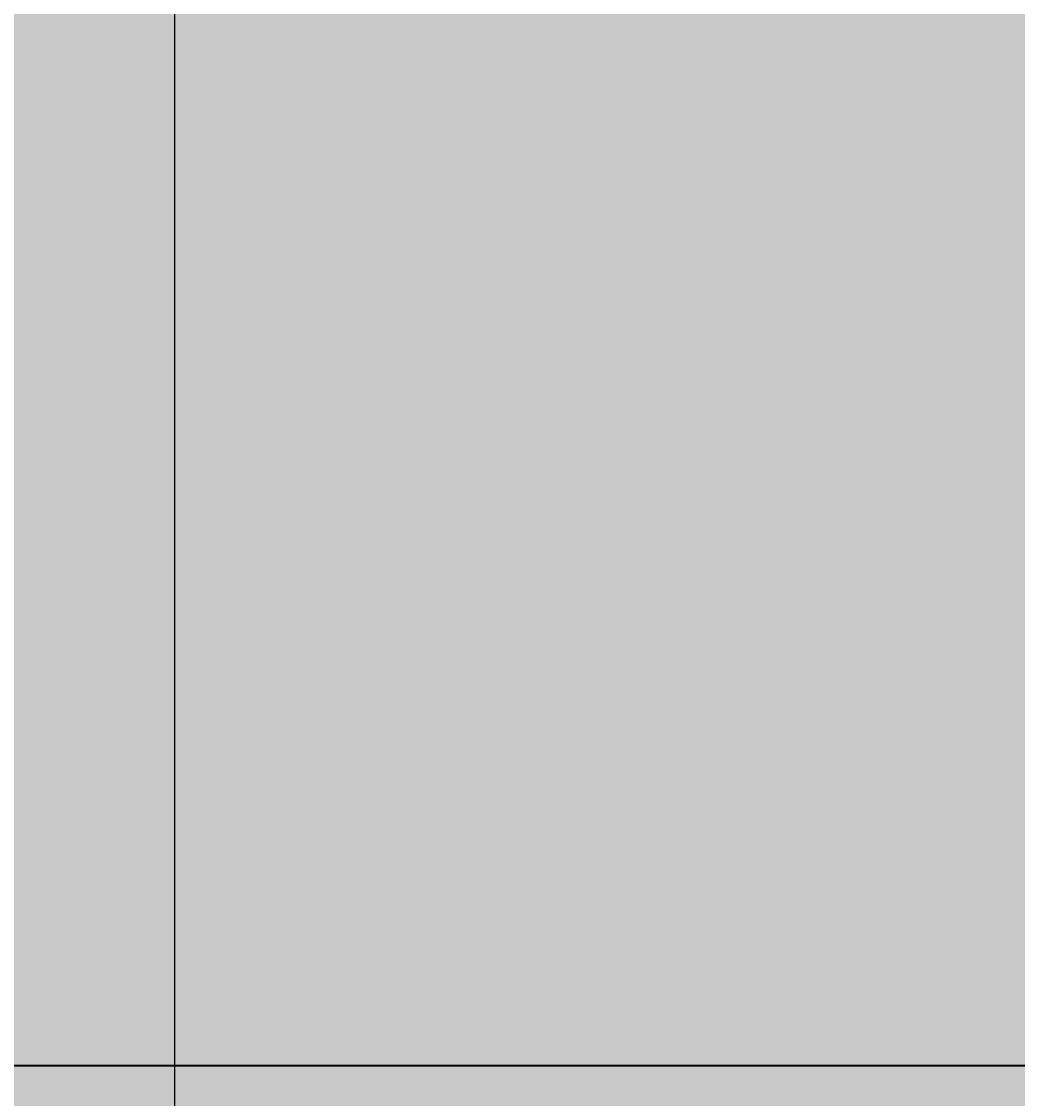
# Model space of a CAD drawing. Units: feet. Extents: x 2695 to 2912, y 795 to 1139.
# Tile 70 of 83: x 2805 to 2840, y 1062 to 1100. Entities that reach past the tile are written whole.
import ezdxf

# ---------------------------------------------------------------- set-up
doc = ezdxf.new("R2010")
doc.units = ezdxf.units.FT
for name, color, linetype, lineweight in [('A-ANNO-DIMS', 2, 'Continuous', 18), ('A-ELEV', 7, 'Continuous', 35), ('A-ELEV-PATT', 252, 'Continuous', 13)]:
    doc.layers.add(name, color=color, linetype=linetype, lineweight=lineweight)
doc.styles.get("Standard").update_dxf_attribs({"font": 'arial.ttf'})
doc.dimstyles.get("Standard").update_dxf_attribs({"dimtxt": 0.18, "dimasz": 0.18, "dimexe": 0.18, "dimexo": 0.0625, "dimgap": 0.09, "dimtad": 0, "dimtih": 1, "dimtoh": 1, "dimdec": 1, "dimzin": 0, "dimdsep": 46, "dimlunit": 3, "dimtxsty": 'Standard', "dimcen": 0.09, "dimadec": 0, "dimazin": 0, "dimtfac": 1, "dimtdec": 1, "dimtofl": 0, "dimtmove": 0, "dimatfit": 3, "dimfxl": 1, "dimtolj": 1, "dimtzin": 0, "dimarcsym": 0})

# ---------------------------------------------------------------- blocks, each defined once
blk = doc.blocks.new('*D10')
at = {"layer": 'A-ANNO-DIMS', "color": 0, "lineweight": -2, "transparency": 16777216}
for p, q in [((2778.034, 1020.886), (2778.034, 1138.886)), ((2778.214, 1138.706), (2810.411, 1138.706)), ((2843.395, 1138.706), (2811.198, 1138.706)), ((2843.575, 1020.886), (2843.575, 1138.886))]:
    blk.add_line(p, q, dxfattribs=at)
at = {"layer": 'A-ANNO-DIMS', "color": 0, "transparency": 16777216}
for points in [[(2778.214, 1138.736), (2778.214, 1138.676), (2778.034, 1138.706)], [(2843.395, 1138.736), (2843.395, 1138.676), (2843.575, 1138.706)]]:
    blk.add_solid(points, dxfattribs=at)
at = {"layer": 'Defpoints', "color": 0, "transparency": 16777216}
for p in [(2843.575, 1138.706), (2778.034, 1020.824), (2843.575, 1020.824)]:
    blk.add_point(p, dxfattribs=at)
at = {"layer": 'A-ANNO-DIMS', "color": 0, "transparency": 16777216, "insert": (2810.805, 1138.706), "char_height": 0.18, "attachment_point": 5}
blk.add_mtext('\\A1;65.54', dxfattribs=at)
blk = doc.blocks.new('*D49')
at = {"layer": 'A-ANNO-DIMS', "color": 0, "lineweight": -2, "transparency": 16777216}
for p, q in [((2772.522, 972.03), (2772.522, 1138.886)), ((2772.702, 1138.706), (2790.888, 1138.706)), ((2809.861, 1138.706), (2791.674, 1138.706)), ((2810.041, 972.03), (2810.041, 1138.886))]:
    blk.add_line(p, q, dxfattribs=at)
at = {"layer": 'A-ANNO-DIMS', "color": 0, "transparency": 16777216}
for points in [[(2772.702, 1138.736), (2772.702, 1138.676), (2772.522, 1138.706)], [(2809.861, 1138.736), (2809.861, 1138.676), (2810.041, 1138.706)]]:
    blk.add_solid(points, dxfattribs=at)
at = {"layer": 'Defpoints', "color": 0, "transparency": 16777216}
for p in [(2810.041, 1138.706), (2772.522, 971.967), (2810.041, 971.967)]:
    blk.add_point(p, dxfattribs=at)
at = {"layer": 'A-ANNO-DIMS', "color": 0, "transparency": 16777216, "insert": (2791.281, 1138.706), "char_height": 0.18, "attachment_point": 5}
blk.add_mtext('\\A1;37.52', dxfattribs=at)
blk = doc.blocks.new('*D50')
at = {"layer": 'A-ANNO-DIMS', "color": 0, "lineweight": -2, "transparency": 16777216}
for p, q in [((2810.041, 972.03), (2810.041, 1138.886)), ((2810.221, 1138.706), (2848.721, 1138.706)), ((2888.008, 1138.706), (2849.508, 1138.706)), ((2888.188, 972.03), (2888.188, 1138.886))]:
    blk.add_line(p, q, dxfattribs=at)
at = {"layer": 'A-ANNO-DIMS', "color": 0, "transparency": 16777216}
for points in [[(2810.221, 1138.736), (2810.221, 1138.676), (2810.041, 1138.706)], [(2888.008, 1138.736), (2888.008, 1138.676), (2888.188, 1138.706)]]:
    blk.add_solid(points, dxfattribs=at)
at = {"layer": 'Defpoints', "color": 0, "transparency": 16777216}
for p in [(2888.188, 1138.706), (2810.041, 971.967), (2888.188, 971.967)]:
    blk.add_point(p, dxfattribs=at)
at = {"layer": 'A-ANNO-DIMS', "color": 0, "transparency": 16777216, "insert": (2849.114, 1138.706), "char_height": 0.18, "attachment_point": 5}
blk.add_mtext('\\A1;78.15', dxfattribs=at)

msp = doc.modelspace()

# ---------------------------------------------------------------- hatches: boundary and pattern name
at = {"layer": 'A-ELEV-PATT'}
h = msp.add_hatch(color=256, dxfattribs=at)
h.set_gradient(color1=(255, 255, 255), tint=1)
h.paths.add_polyline_path([(2770.6361, 1122.9306), (2710.6361, 1122.9306), (2710.6361, 1118.4096), (2770.6361, 1118.4096)])
h.paths.add_polyline_path([(2890.6361, 1107.8588), (2770.6361, 1107.8588), (2770.6361, 1103.3378), (2890.6361, 1103.3378)])
h.paths.add_polyline_path([(2890.6361, 1062.9306), (2710.6361, 1062.9306), (2710.6361, 1056.9306), (2710.6361, 936.9306), (2710.6361, 924.3105), (2716.5358, 924.3105), (2890.6361, 924.3105), (2890.6361, 936.9306), (2715.8852, 936.9306), (2715.8852, 1050.3105), (2890.6361, 1050.3105)])
h.paths.add_polyline_path([(2716.5358, 924.3105), (2710.6361, 924.3105), (2710.6361, 810.9306), (2716.5358, 810.9306)])
h = msp.add_hatch(color=256, dxfattribs=at)
h.set_gradient(color1=(147, 149, 152), color2=(147, 149, 152), tint=1)
h.paths.add_polyline_path([(2770.6361, 1118.4096), (2710.6361, 1118.4096), (2710.6361, 1062.9306), (2770.6361, 1062.9306)])
h.paths.add_polyline_path([(2890.6361, 1103.3378), (2770.6361, 1103.3378), (2770.6361, 1062.9306), (2890.6361, 1062.9306)])
h.paths.add_polyline_path([(2730.7081, 1048.1052), (2755.1125, 1048.1052), (2755.1125, 936.9306), (2770.6361, 936.9306), (2770.6361, 1050.3105), (2715.8852, 1050.3105), (2715.8852, 936.9306), (2730.7081, 936.9306)])
h.paths.add_polyline_path([(2890.6361, 1050.3105), (2770.6361, 1050.3105), (2770.6361, 971.9673), (2778.0341, 971.9673), (2778.0341, 1020.8235), (2843.575, 1020.8235), (2843.575, 971.9673), (2890.6361, 971.9673)])
h.paths.add_polyline_path([(2888.1882, 970.7156), (2843.575, 970.7156), (2843.575, 964.8267), (2888.1882, 964.8267)])
h.paths.add_polyline_path([(2888.1882, 964.1328), (2843.575, 964.1328), (2843.575, 956.614), (2888.1882, 956.614)])
h.paths.add_polyline_path([(2888.1882, 955.9202), (2843.575, 955.9202), (2843.575, 949.2892), (2888.1882, 949.2892)])
h.paths.add_polyline_path([(2888.1882, 948.5954), (2843.575, 948.5954), (2843.575, 941.3507), (2888.1882, 941.3507)])
h.paths.add_polyline_path([(2888.1882, 940.6569), (2843.575, 940.6569), (2843.575, 936.9306), (2888.1882, 936.9306)])
h.paths.add_polyline_path([(2890.6361, 970.7156), (2888.9368, 970.7156), (2888.9368, 964.8267), (2890.6361, 964.8267)])
h.paths.add_polyline_path([(2890.6361, 964.1328), (2888.9368, 964.1328), (2888.9368, 956.614), (2890.6361, 956.614)])
h.paths.add_polyline_path([(2890.6361, 955.9202), (2888.9368, 955.9202), (2888.9368, 949.2892), (2890.6361, 949.2892)])
h.paths.add_polyline_path([(2890.6361, 940.6569), (2888.9368, 940.6569), (2888.9368, 936.9306), (2890.6361, 936.9306)])
h.paths.add_polyline_path([(2890.6361, 948.5954), (2888.9368, 948.5954), (2888.9368, 941.3507), (2890.6361, 941.3507)])
h.paths.add_polyline_path([(2772.5216, 970.7156), (2770.6361, 970.7156), (2770.6361, 964.8267), (2772.5216, 964.8267)])
h.paths.add_polyline_path([(2772.5216, 964.1328), (2770.6361, 964.1328), (2770.6361, 956.614), (2772.5216, 956.614)])
h.paths.add_polyline_path([(2772.5216, 955.9202), (2770.6361, 955.9202), (2770.6361, 949.2892), (2772.5216, 949.2892)])
h.paths.add_polyline_path([(2772.5216, 948.5954), (2770.6361, 948.5954), (2770.6361, 941.3507), (2772.5216, 941.3507)])
h.paths.add_polyline_path([(2772.5216, 940.6569), (2770.6361, 940.6569), (2770.6361, 936.9306), (2772.5216, 936.9306)])
h.paths.add_polyline_path([(2778.0341, 940.6569), (2773.2702, 940.6569), (2773.2702, 936.9306), (2778.0341, 936.9306)])
h.paths.add_polyline_path([(2778.0341, 970.7156), (2773.2702, 970.7156), (2773.2702, 964.8267), (2778.0341, 964.8267)])
h.paths.add_polyline_path([(2778.0341, 964.1328), (2773.2702, 964.1328), (2773.2702, 956.614), (2778.0341, 956.614)])
h.paths.add_polyline_path([(2778.0341, 955.9202), (2773.2702, 955.9202), (2773.2702, 949.2892), (2778.0341, 949.2892)])
h.paths.add_polyline_path([(2778.0341, 948.5954), (2773.2702, 948.5954), (2773.2702, 941.3507), (2778.0341, 941.3507)])
h.paths.add_polyline_path([(2810.0407, 940.6569), (2780.0341, 940.6569), (2780.0341, 936.9306), (2810.0407, 936.9306)])
h.paths.add_polyline_path([(2890.6361, 924.3105), (2770.6361, 924.3105), (2770.6361, 810.9306), (2773.5029, 810.9306), (2773.5029, 905.5143), (2805.9398, 905.5143), (2838.3767, 905.5143), (2838.3767, 810.9306), (2890.6361, 810.9306)])
h = msp.add_hatch(color=256, dxfattribs=at)
h.set_gradient(color1=(199, 200, 202), color2=(213, 227, 240), centered=1)
h.paths.add_polyline_path([(2890.6361, 1103.3378), (2770.6361, 1103.3378), (2770.6361, 1062.9306), (2890.6361, 1062.9306)])

# ---------------------------------------------------------------- linework, layer by layer
at = {"layer": 'A-ELEV'}
for q in [(2890.6361, 1062.9306), (2895.4694, 1062.9306)]:
    msp.add_line((2710.6361, 1062.9306), q, dxfattribs=at)

# ---------------------------------------------------------------- dimensions: what is measured, and where the dimension line sits
at = {"layer": 'A-ANNO-DIMS'}
for base, p1, p2, picture, middle in [((2810.0407, 1138.7056), (2772.5216, 971.9673), (2810.0407, 971.9673), '*D49', (2791.2811, 1138.7056)), ((2843.575, 1138.7056), (2778.0341, 1020.8235), (2843.575, 1020.8235), '*D10', (2810.8045, 1138.7056)), ((2888.1882, 1138.7056), (2810.0407, 971.9673), (2888.1882, 971.9673), '*D50', (2849.1144, 1138.7056))]:
    dim = msp.add_linear_dim(base=base, p1=p1, p2=p2, dimstyle='Standard', override={"dimdec": 2, "dimlfac": 1, "dimrnd": 0, "dimzin": 0, "dimdsep": 46, "dimlunit": 2}, dxfattribs=at)
    dim.commit()
    dim.dimension.update_dxf_attribs({"geometry": picture, "text_midpoint": middle})

doc.saveas('drawing.dxf')
